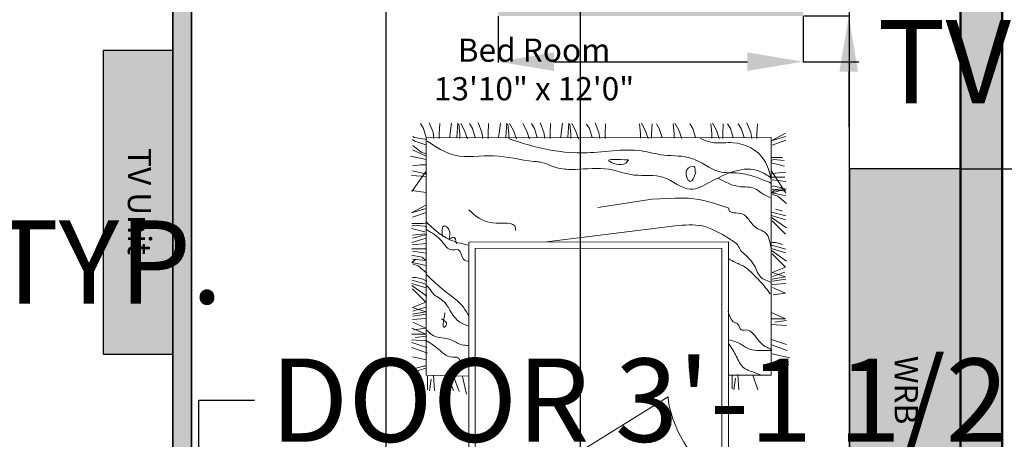
# Model space of a CAD drawing. Units: inches. Extents: x 2796 to 3603, y 978 to 1787.
# Tile 13 of 15: x 3212 to 3425, y 1545 to 1636. Entities that reach past the tile are written whole.
import ezdxf

# ---------------------------------------------------------------- set-up
doc = ezdxf.new("R2010")
doc.units = ezdxf.units.IN
for name, color, linetype, lineweight in [('A-ANNO-DIMS', 7, 'Continuous', 18), ('A-ANNO-TEXT', 7, 'Continuous', 18), ('A-AREA-IDEN', 7, 'Continuous', 18), ('A-FLOR-CASE', 2, 'Continuous', 25), ('A-FLOR-CASE-PATT', 2, 'Continuous', 13), ('A-WALL-EXTR-PATT', 1, 'Continuous', 13), ('A-WALL-INTR-PATT', 5, 'Continuous', 13), ('Furniture', 2, 'Continuous', 18), ('Inner Wall', 5, 'Continuous', 35), ('Outer Wall', 1, 'Continuous', 50)]:
    doc.layers.add(name, color=color, linetype=linetype, lineweight=lineweight)
doc.styles.get("Standard").update_dxf_attribs({"font": 'arial.ttf'})
doc.dimstyles.get("Standard").update_dxf_attribs({"dimtxt": 18, "dimasz": 12, "dimexe": 0.18, "dimexo": 0.0625, "dimgap": 0.09, "dimtad": 0, "dimtih": 1, "dimtoh": 1, "dimdec": 0, "dimzin": 0, "dimdsep": 46, "dimlunit": 3, "dimtxsty": 'Standard', "dimcen": 0.09, "dimadec": 0, "dimazin": 0, "dimtfac": 1, "dimtdec": 0, "dimtofl": 0, "dimtmove": 0, "dimatfit": 3, "dimfxl": 1, "dimtolj": 1, "dimtzin": 0, "dimarcsym": 0})

# ---------------------------------------------------------------- blocks, each defined once
blk = doc.blocks.new('A$C2B723114')
for p, q in [((0, 2.9047), (2.8274, 2.9047)), ((0, 2.8487), (0, 2.9047)), ((0.4243, 2.8697), (0.4243, 2.4855)), ((2.4742, 2.8697), (2.4742, 2.4855)), ((2.8274, 2.9047), (2.8274, 2.8487)), ((2.8274, 2.8487), (0, 2.8487)), ((0.1012, 2.4649), (0.1012, 2.849)), ((0.1396, 2.5033), (0.1396, 2.849)), ((0.6794, 0.7051), (0.6794, 2.8509)), ((0.7187, 0.7435), (0.7187, 2.8509)), ((2.1776, 2.8509), (2.1776, 0.7454)), ((2.216, 2.8509), (2.216, 0.707)), ((2.6798, 2.5052), (2.6798, 2.8509)), ((2.7182, 2.4668), (2.7182, 2.8509)), ((0.6087, 2.6776), (0.295, 2.6776)), ((2.6586, 2.6776), (2.2821, 2.6776)), ((1.3789, 2.4999), (1.3598, 2.5761)), ((2.0593, 2.4999), (2.0402, 2.5761)), ((2.2188, 2.5052), (2.6798, 2.5052)), ((0.6794, 2.4649), (0.1012, 2.4649)), ((0.6766, 2.5033), (0.1396, 2.5033)), ((0.7191, 2.47), (2.1778, 2.4719)), ((1.3858, 2.4723), (1.3789, 2.4999)), ((2.0662, 2.4723), (2.0593, 2.4999)), ((2.2188, 2.4668), (2.7182, 2.4668)), ((2.1771, 2.3036), (0.718, 2.1685)), ((1.0365, 1.6233), (2.1246, 2.2989)), ((0.5047, 1.5819), (0.5353, 1.4945)), ((0.6174, 1.5819), (0.6232, 1.4916)), ((0.6467, 1.5819), (0.6369, 1.5137)), ((0.6571, 1.4945), (0.6571, 1.5765)), ((2.2287, 1.6076), (2.2523, 1.5035)), ((2.2726, 1.593), (2.3061, 1.5007)), ((2.3067, 1.5881), (2.3373, 1.5007)), ((2.4194, 1.5881), (2.4251, 1.4979)), ((2.4487, 1.5881), (2.4389, 1.5199)), ((2.4591, 1.5007), (2.4591, 1.5828)), ((0.4269, 0.0884), (0.4269, 1.4945)), ((0.4269, 1.4945), (0.6794, 1.4945)), ((2.4685, 1.4964), (2.216, 1.5022)), ((2.4685, 1.4964), (2.4685, 0.0903)), ((2.4685, 1.4044), (2.5491, 1.3861)), ((0.3172, 1.3923), (0.4213, 1.3687)), ((0.3318, 1.3485), (0.4241, 1.3149)), ((2.4596, 1.3659), (2.552, 1.3324)), ((0.3367, 1.3143), (0.4241, 1.2838)), ((2.4645, 1.3318), (2.552, 1.3012)), ((2.4645, 1.2928), (2.5548, 1.2871)), ((2.4645, 1.2635), (2.5328, 1.2733)), ((2.4699, 1.2531), (2.552, 1.2163)), ((2.552, 1.2531), (2.4699, 1.2531)), ((2.5435, 1.2276), (2.4699, 1.2163)), ((0.3367, 1.2016), (0.427, 1.1959)), ((0.3367, 1.1724), (0.405, 1.1821)), ((2.5491, 1.1654), (2.467, 1.1597)), ((2.4699, 1.2163), (2.5463, 1.1823)), ((0.4241, 1.162), (0.3421, 1.162)), ((0.3421, 1.162), (0.4241, 1.1252)), ((2.5463, 1.1455), (2.467, 1.1342)), ((2.5491, 1.1342), (2.4699, 1.1201)), ((2.4699, 1.1201), (2.5491, 1.0946)), ((2.5463, 1.1172), (2.4727, 1.0918)), ((2.5491, 1.0946), (2.4699, 1.0635)), ((2.4699, 1.0635), (2.5491, 0.9842)), ((0.4157, 1.0206), (0.3421, 1.0093)), ((0.3421, 1.0093), (0.4185, 0.9754)), ((2.4642, 1.0267), (2.552, 0.9644)), ((0.4213, 0.9584), (0.3392, 0.9527)), ((0.4185, 0.9386), (0.3392, 0.9272)), ((2.4642, 0.9389), (2.4869, 0.9276)), ((2.467, 0.9559), (2.552, 0.9333)), ((2.4699, 0.9785), (2.552, 0.9531)), ((0.4213, 0.9272), (0.3421, 0.9131)), ((0.3421, 0.9131), (0.4213, 0.8876)), ((0.4213, 0.8876), (0.3421, 0.8565)), ((0.4185, 0.9103), (0.3449, 0.8848)), ((2.4642, 0.8908), (2.5152, 0.8483)), ((2.4869, 0.9276), (2.5265, 0.9163)), ((2.5265, 0.9163), (2.5491, 0.9163)), ((0.3364, 0.8197), (0.4241, 0.7574)), ((0.3421, 0.8565), (0.4213, 0.7772)), ((2.467, 0.8455), (2.5208, 0.8342)), ((2.4699, 0.8172), (2.4925, 0.7974)), ((2.5491, 0.8087), (2.4699, 0.8172)), ((2.5152, 0.8483), (2.5491, 0.837)), ((2.5208, 0.8342), (2.552, 0.8285)), ((2.552, 0.8285), (2.5293, 0.8087)), ((0.3421, 0.7716), (0.4241, 0.7461)), ((2.5491, 0.7606), (2.467, 0.7719)), ((2.4925, 0.7974), (2.535, 0.7889)), ((2.535, 0.7889), (2.552, 0.7861)), ((0.3392, 0.7489), (0.4241, 0.7263)), ((0.359, 0.7206), (0.3987, 0.7093)), ((0.3987, 0.7093), (0.4213, 0.7093)), ((2.216, 0.707), (0.6794, 0.7051)), ((2.1776, 0.7454), (0.7187, 0.7435)), ((0.9938, 0.6115), (1.7555, 0.7064)), ((2.4727, 0.7464), (2.467, 0.7408)), ((2.467, 0.7153), (2.5491, 0.7238)), ((2.552, 0.7096), (2.467, 0.6842)), ((2.552, 0.7464), (2.4727, 0.7464)), ((0.3421, 0.6601), (0.4213, 0.5808)), ((2.5491, 0.6842), (2.4642, 0.6615)), ((2.5491, 0.6672), (2.4755, 0.6587)), ((2.4755, 0.6474), (2.5548, 0.6276)), ((0.3364, 0.6233), (0.4241, 0.561)), ((2.4642, 0.6191), (2.4784, 0.6134)), ((2.467, 0.5993), (2.4869, 0.5964)), ((2.4784, 0.6134), (2.5406, 0.6077)), ((2.4869, 0.5964), (2.552, 0.5964)), ((2.5406, 0.6077), (2.552, 0.6134)), ((0.3392, 0.5525), (0.4241, 0.5299)), ((0.3421, 0.5752), (0.4241, 0.5497)), ((2.467, 0.5313), (2.5491, 0.5596)), ((2.467, 0.5087), (2.5548, 0.5342)), ((2.5548, 0.5342), (2.4699, 0.4889)), ((0.3364, 0.4785), (0.3874, 0.436)), ((0.359, 0.5242), (0.3987, 0.5129)), ((1.4523, 0.5021), (1.1305, 0.4537)), ((0.4213, 0.415), (0.3364, 0.3923)), ((0.3392, 0.4332), (0.393, 0.4219)), ((0.4241, 0.2868), (0.3392, 0.415)), ((0.3874, 0.436), (0.4213, 0.4247)), ((0.393, 0.4219), (0.4241, 0.4162)), ((0.4241, 0.4162), (0.4015, 0.3964)), ((1.1305, 0.4537), (0.9938, 0.448)), ((2.467, 0.4133), (2.552, 0.4019)), ((0.3421, 0.4049), (0.3647, 0.3851)), ((0.4213, 0.3964), (0.3421, 0.4049)), ((0.4213, 0.398), (0.3477, 0.3895)), ((0.3647, 0.3851), (0.4072, 0.3766)), ((0.4072, 0.3766), (0.4241, 0.3738)), ((2.467, 0.2879), (2.552, 0.4076)), ((0.4213, 0.3377), (0.3392, 0.3491)), ((0.3392, 0.2925), (0.4213, 0.3009)), ((0.4241, 0.3236), (0.3449, 0.3236)), ((2.4642, 0.3049), (2.5491, 0.2851)), ((2.467, 0.319), (2.5548, 0.3134)), ((0.3477, 0.2571), (0.427, 0.2373)), ((2.4699, 0.2491), (2.501, 0.2491)), ((2.501, 0.2491), (2.5491, 0.2547)), ((0.3506, 0.2231), (0.4128, 0.2175)), ((0.359, 0.2061), (0.4241, 0.2061)), ((0.4128, 0.2175), (0.4241, 0.2231)), ((2.467, 0.2179), (2.5605, 0.1981)), ((2.467, 0.1981), (2.5491, 0.1613)), ((2.467, 0.184), (2.4982, 0.1755)), ((2.4982, 0.1755), (2.5463, 0.1359)), ((0.3392, 0.1042), (0.4213, 0.1325)), ((2.4699, 0.1302), (2.535, 0.1104)), ((0.3392, 0.0815), (0.427, 0.107)), ((0.427, 0.107), (0.3421, 0.0617)), ((2.4685, 0.0903), (0.4269, 0.0884)), ((0.5106, 0.0657), (0.5077, 0.0063)), ((0.5106, 0.094), (0.5106, 0.0657)), ((0.5417, 0.094), (0.5474, 0.0572)), ((0.587, 0.0884), (0.604, 0.0346)), ((0.6512, 0.0884), (0.6682, 0.0346)), ((0.713, 0.0657), (0.7101, 0.0063)), ((0.713, 0.094), (0.713, 0.0657)), ((0.7334, 0.0943), (0.7503, 0.0434)), ((0.7786, 0.0915), (0.7786, 0.0632)), ((0.7786, 0.0632), (0.7843, 0.0066)), ((0.8739, 0.0884), (0.8908, 0.0346)), ((0.956, 0.0943), (0.973, 0.0434)), ((1.0013, 0.0915), (1.0013, 0.0632)), ((1.0013, 0.0632), (1.007, 0.0066)), ((1.072, 0.0884), (1.089, 0.0346)), ((1.1338, 0.0657), (1.131, 0.0063)), ((1.1338, 0.094), (1.1338, 0.0657)), ((1.1542, 0.0943), (1.1712, 0.0434)), ((1.1995, 0.0915), (1.1995, 0.0632)), ((1.1995, 0.0632), (1.2052, 0.0066)), ((1.4088, 0.0657), (1.406, 0.0063)), ((1.4088, 0.094), (1.4088, 0.0657)), ((1.44, 0.094), (1.4456, 0.0572)), ((1.4853, 0.0884), (1.5023, 0.0346)), ((1.5674, 0.0962), (1.5844, 0.0453)), ((1.6127, 0.0934), (1.6127, 0.0651)), ((1.6127, 0.0651), (1.6184, 0.0085)), ((1.6297, 0.0849), (1.624, 0.0028)), ((1.6693, 0.0623), (1.6608, 0.0028)), ((1.6721, 0.0877), (1.6693, 0.0623)), ((1.7344, 0.0651), (1.7316, 0.0057)), ((1.7344, 0.0934), (1.7344, 0.0651)), ((1.7655, 0.0934), (1.7712, 0.0566)), ((1.8108, 0.0877), (1.8278, 0.034)), ((1.8568, 0.0962), (1.8738, 0.0453)), ((1.9342, 0.0962), (1.9512, 0.0453)), ((1.9795, 0.0934), (1.9795, 0.0651)), ((1.9795, 0.0651), (1.9852, 0.0085)), ((1.9965, 0.0849), (1.9908, 0.0028)), ((2.0361, 0.0623), (2.0276, 0.0028)), ((2.039, 0.0877), (2.0361, 0.0623)), ((2.1012, 0.0651), (2.0984, 0.0057)), ((2.1012, 0.0934), (2.1012, 0.0651)), ((2.1324, 0.0934), (2.138, 0.0566)), ((2.1777, 0.0877), (2.1946, 0.034)), ((2.2236, 0.0962), (2.2406, 0.0453)), ((2.2689, 0.0934), (2.2689, 0.0651)), ((2.2689, 0.0651), (2.2746, 0.0085)), ((2.2859, 0.0849), (2.2802, 0.0028)), ((2.3255, 0.0623), (2.317, 0.0028)), ((2.3284, 0.0877), (2.3255, 0.0623)), ((2.3906, 0.0651), (2.3878, 0.0057)), ((2.3906, 0.0934), (2.3906, 0.0651)), ((2.4218, 0.0934), (2.4274, 0.0566)), ((2.4642, 0.0991), (2.5378, 0.0877)), ((2.467, 0.0877), (2.484, 0.034)), ((2.535, 0.1104), (2.5491, 0.0991)), ((2.5378, 0.0877), (2.5463, 0.0821)), ((0.5474, 0.0572), (0.57, 0.0006)), ((0.604, 0.0346), (0.621, 0.0063)), ((0.6682, 0.0346), (0.6851, 0.0063)), ((0.7503, 0.0434), (0.773, 0.0037)), ((0.8908, 0.0346), (0.9078, 0.0063)), ((0.973, 0.0434), (0.9957, 0.0037)), ((1.089, 0.0346), (1.106, 0.0063)), ((1.1712, 0.0434), (1.1939, 0.0037)), ((1.4456, 0.0572), (1.4683, 0.0006)), ((1.5023, 0.0346), (1.5192, 0.0082)), ((1.5844, 0.0453), (1.607, 0.0057)), ((1.7712, 0.0566), (1.7938, 0)), ((1.8278, 0.034), (1.8448, 0.0057)), ((1.8738, 0.0453), (1.8964, 0.0057)), ((1.9512, 0.0453), (1.9739, 0.0057)), ((2.138, 0.0566), (2.1607, 0)), ((2.1946, 0.034), (2.2116, 0.0057)), ((2.2406, 0.0453), (2.2632, 0.0057)), ((2.4274, 0.0566), (2.4501, 0)), ((2.484, 0.034), (2.501, 0.0057))]:
    blk.add_line(p, q)
for centre, radius in [((0.4243, 2.6776), 0.0821), ((2.4742, 2.6776), 0.0821), ((0.4243, 2.6776), 0.0493), ((2.4742, 2.6776), 0.0493)]:
    blk.add_circle(centre, radius)
for centre, radius, start, end in [((0.8078, 2.821), 0.00214, 160.43603, 281.89306), ((0.8088, 2.8207), 0.00315, 111.7883, 160.43603), ((0.8162, 2.8021), 0.0232, 94.30254, 111.7883), ((0.8091, 2.8151), 0.00394, 21.9904, 101.89306), ((0.8409, 2.7949), 0.0302, 158.57902, 188.13348), ((0.7994, 2.8112), 0.0144, 338.57902, 21.9904), ((0.8165, 2.7987), 0.0266, 59.34875, 94.30254), ((0.8554, 2.8643), 0.0497, 239.34875, 264.74081), ((0.9202, 3.5684), 0.7568, 264.74081, 268.09211), ((0.8679, 2.7254), 0.0915, 74.06476, 94.21588), ((0.8679, 2.7254), 0.0915, 53.91364, 74.06476), ((0.9409, 4.189), 1.3777, 268.09211, 270.57574), ((0.8679, 2.7254), 0.0915, 36.17665, 53.91364), ((0.86, 2.6097), 0.2158, 62.76041, 69.13972), ((0.9466, 3.6164), 0.8051, 270.57574, 274.80185), ((0.9263, 2.7386), 0.0708, 51.61143, 62.76041), ((1.0364, 2.548), 0.2671, 87.46141, 94.80185), ((1.042, 2.6745), 0.1405, 79.81012, 87.46141), ((1.1532, 3.2931), 0.488, 259.81012, 263.9133), ((1.204, 3.7695), 0.9671, 263.9133, 270), ((1.204, 3.4318), 0.6294, 270, 277.54685), ((1.2573, 3.0292), 0.2233, 277.54685, 285.74398), ((1.3941, 2.5438), 0.281, 98.43719, 105.74398), ((1.3747, 2.6748), 0.1486, 90, 98.43719), ((1.3713, 2.8186), 0.0315, 274.40021, 333.41948), ((1.3747, 2.74), 0.0833, 78.72762, 90), ((1.3886, 2.8099), 0.0121, 333.41948, 78.72762), ((1.4882, 2.821), 0.00214, 160.43603, 281.89306), ((1.4892, 2.8207), 0.00315, 111.7883, 160.43603), ((1.4966, 2.8021), 0.0232, 94.30254, 111.7883), ((1.4895, 2.8151), 0.00394, 21.9904, 101.89306), ((1.5213, 2.7949), 0.0302, 158.57902, 188.13348), ((1.4798, 2.8112), 0.0144, 338.57902, 21.9904), ((1.4969, 2.7987), 0.0266, 59.34875, 94.30254), ((1.5358, 2.8643), 0.0497, 239.34875, 264.74081), ((1.6006, 3.5684), 0.7568, 264.74081, 268.09211), ((1.5483, 2.7254), 0.0915, 74.06476, 94.21588), ((1.5483, 2.7254), 0.0915, 53.91364, 74.06476), ((1.6213, 4.189), 1.3777, 268.09211, 270.57574), ((1.5483, 2.7254), 0.0915, 36.17665, 53.91364), ((1.5404, 2.6097), 0.2158, 62.76041, 69.13972), ((1.627, 3.6164), 0.8051, 270.57574, 274.80185), ((1.6067, 2.7386), 0.0708, 51.61143, 62.76041), ((1.7168, 2.548), 0.2671, 87.46141, 94.80185), ((1.7224, 2.6745), 0.1405, 79.81012, 87.46141), ((1.8336, 3.2931), 0.488, 259.81012, 263.9133), ((1.8844, 3.7695), 0.9671, 263.9133, 270), ((1.8844, 3.4318), 0.6294, 270, 277.54685), ((1.9377, 3.0292), 0.2233, 277.54685, 285.74398), ((2.0745, 2.5438), 0.281, 98.43719, 105.74398), ((2.0551, 2.6748), 0.1486, 90, 98.43719), ((2.0517, 2.8186), 0.0315, 274.40021, 333.41948), ((2.0551, 2.74), 0.0833, 78.72762, 90), ((2.069, 2.8099), 0.0121, 333.41948, 78.72762), ((1.0356, 2.8227), 0.2268, 188.13348, 192.10946), ((0.635, 2.7368), 0.1829, 7.6809, 12.10946), ((-0.0181, 2.6487), 0.8418, 3.36875, 7.6809), ((0.8679, 2.7254), 0.0915, 18.43965, 36.17665), ((0.7461, 2.511), 0.3611, 46.18849, 51.61143), ((0.8523, 2.6218), 0.2076, 39.03494, 46.18849), ((0.9783, 2.7239), 0.0455, 28.31676, 39.03494), ((0.8558, 2.6579), 0.1846, 23.00277, 28.31676), ((0.923, 2.7382), 0.4535, 0, 6.23236), ((1.1884, 2.7382), 0.1881, 350.31563, 0), ((1.716, 2.8227), 0.2268, 188.13348, 192.10946), ((1.3154, 2.7368), 0.1829, 7.6809, 12.10946), ((0.6623, 2.6487), 0.8418, 3.36875, 7.6809), ((1.5483, 2.7254), 0.0915, 18.43965, 36.17665), ((1.4265, 2.511), 0.3611, 46.18849, 51.61143), ((1.5327, 2.6218), 0.2076, 39.03494, 46.18849), ((1.6587, 2.7239), 0.0455, 28.31676, 39.03494), ((1.5362, 2.6579), 0.1846, 23.00277, 28.31676), ((1.6034, 2.7382), 0.4535, 0, 6.23236), ((1.8688, 2.7382), 0.1881, 350.31563, 0), ((0.1976, 2.6614), 0.6258, 358.36691, 3.36875), ((0.5722, 2.8434), 0.8132, 347.80162, 350.31563), ((0.878, 2.6614), 0.6258, 358.36691, 3.36875), ((1.2526, 2.8434), 0.8132, 347.80162, 350.31563), ((-0.4351, 2.6794), 1.2587, 356.94504, 358.36691), ((1.9648, 2.5659), 0.6074, 171.99495, 177.33512), ((1.6528, 2.6098), 0.2924, 167.80162, 171.99495), ((0.2453, 2.6794), 1.2587, 356.94504, 358.36691), ((2.6452, 2.5659), 0.6074, 171.99495, 177.33512), ((2.3332, 2.6098), 0.2924, 167.80162, 171.99495), ((-11.7321, 3.2823), 12.5718, 356.49514, 356.94504), ((1.4204, 2.5912), 0.0624, 177.33512, 194.04519), ((-11.0517, 3.2823), 12.5718, 356.49514, 356.94504), ((2.1008, 2.5912), 0.0624, 177.33512, 194.04519), ((0.5206, 2.5319), 0.2961, 350.00164, 356.49514), ((1.4917, 3.1364), 0.681, 244.68893, 246.51559), ((1.4917, 3.1364), 0.681, 246.51559, 248.34226), ((1.201, 2.5319), 0.2961, 350.00164, 356.49514), ((2.1721, 3.1364), 0.681, 244.68893, 246.51559), ((2.1721, 3.1364), 0.681, 246.51559, 248.34226), ((0.8298, 2.4774), 0.0178, 170.00164, 196.69777), ((0.8139, 2.4726), 0.00122, 196.69777, 277.12039), ((0.8041, 2.5514), 0.0807, 277.12039, 286.22115), ((0.8068, 2.5419), 0.0707, 286.22115, 297.28412), ((0.8584, 2.4419), 0.0418, 102.86904, 117.28412), ((0.879, 2.3515), 0.1345, 93.57397, 102.86904), ((0.9376, 1.4146), 1.0732, 90.28654, 93.57397), ((0.9586, -2.7845), 5.2724, 89.02962, 90.28654), ((0.9954, -0.6123), 3.0999, 87.39037, 89.02962), ((1.0854, 1.364), 1.1216, 85.38242, 87.39037), ((1.28, 3.7729), 1.2952, 265.38242, 267.25094), ((1.228, 2.691), 0.2121, 267.25094, 281.55856), ((1.4917, 3.1364), 0.681, 248.34226, 250.57202), ((1.4917, 3.1364), 0.681, 250.57202, 252.80178), ((1.2975, 2.3514), 0.1345, 83.56595, 101.55856), ((1.3002, 2.3754), 0.1104, 72.61359, 83.56595), ((1.3965, 2.6828), 0.2118, 252.61359, 260.5159), ((1.4027, 2.7202), 0.2496, 260.5159, 265.91706), ((1.385, 2.4721), 0.000845, 265.91706, 14.04494), ((1.5102, 2.4774), 0.0178, 170.00164, 196.69777), ((1.4943, 2.4726), 0.00122, 196.69777, 277.12039), ((1.4845, 2.5514), 0.0807, 277.12039, 286.22115), ((1.4872, 2.5419), 0.0707, 286.22115, 297.28412), ((1.5388, 2.4419), 0.0418, 102.86904, 117.28412), ((1.5594, 2.3515), 0.1345, 93.57397, 102.86904), ((1.618, 1.4146), 1.0732, 90.28654, 93.57397), ((1.639, -2.7845), 5.2724, 89.02962, 90.28654), ((1.6758, -0.6123), 3.0999, 87.39037, 89.02962), ((1.7658, 1.364), 1.1216, 85.38242, 87.39037), ((1.9604, 3.7729), 1.2952, 265.38242, 267.25094), ((1.9084, 2.691), 0.2121, 267.25094, 281.55856), ((2.1721, 3.1364), 0.681, 248.34226, 250.57202), ((2.1721, 3.1364), 0.681, 250.57202, 252.80178), ((1.9779, 2.3514), 0.1345, 83.56595, 101.55856), ((1.9806, 2.3754), 0.1104, 72.61359, 83.56595), ((2.0769, 2.6828), 0.2118, 252.61359, 260.5159), ((2.0831, 2.7202), 0.2496, 260.5159, 265.91706), ((2.0654, 2.4721), 0.000845, 265.91706, 14.04494)]:
    blk.add_arc(centre, radius, start, end)
blk.add_ellipse((0.4962, 1.9132), major_axis=(0.4887, -0.4605), ratio=0.503305, start_param=0.491272, end_param=1.591113)
for points, knots in [([(0.427, 1.4678), (0.4036, 1.4582), (0.3693, 1.4441), (0.3335, 1.4344), (0.3221, 1.4313)], [0, 0, 0, 0, 98.452083, 144.639601, 144.639601, 144.639601, 144.639601]), ([(0.6768, 1.3104), (0.6615, 1.3339), (0.6315, 1.3797), (0.604, 1.4501), (0.5417, 1.4748), (0.5064, 1.4871), (0.4848, 1.4945)], [0, 0, 0, 0, 110.980521, 216.571322, 273.316778, 363.252298, 363.252298, 363.252298, 363.252298]), ([(2.5548, 1.4853), (2.5314, 1.4757), (2.5031, 1.4641), (2.4737, 1.4555), (2.4685, 1.454)], [0, 0, 0, 0, 98.452083, 119.481049, 119.481049, 119.481049, 119.481049]), ([(2.552, 1.4598), (2.5309, 1.4545), (2.5031, 1.4475), (2.4753, 1.4406), (2.4685, 1.4389)], [0, 0, 0, 0, 84.638756, 111.94623, 111.94623, 111.94623, 111.94623]), ([(0.4241, 1.4423), (0.4031, 1.437), (0.3691, 1.4284), (0.3351, 1.4199), (0.3221, 1.4167)], [0, 0, 0, 0, 84.638756, 136.955563, 136.955563, 136.955563, 136.955563]), ([(2.2145, 1.4211), (2.233, 1.4246), (2.2636, 1.4303), (2.2761, 1.3837), (2.3429, 1.3967), (2.3949, 1.3342), (2.4474, 1.3031), (2.4698, 1.2898)], [0, 0, 0, 0, 61.886907, 102.717887, 145.699352, 284.082577, 386.765171, 386.765171, 386.765171, 386.765171]), ([(0.6768, 1.286), (0.6567, 1.2911), (0.6145, 1.3017), (0.5543, 1.3533), (0.4816, 1.349), (0.4362, 1.3493), (0.4233, 1.3493)], [0, 0, 0, 0, 80.250278, 168.388677, 295.908361, 346.663112, 346.663112, 346.663112, 346.663112]), ([(0.4233, 1.3445), (0.4367, 1.3385), (0.464, 1.3264), (0.5129, 1.2848), (0.5456, 1.2161), (0.6131, 1.2349), (0.6142, 1.1913), (0.6642, 1.1806), (0.674, 1.144), (0.6817, 1.1154)], [0, 0, 0, 0, 56.745495, 115.23739, 254.956954, 286.678662, 337.828324, 366.201072, 468.500395, 468.500395, 468.500395, 468.500395]), ([(2.2145, 1.319), (2.2295, 1.319), (2.2678, 1.3192), (2.3288, 1.2705), (2.4143, 1.279), (2.4535, 1.2403), (2.4662, 1.2278)], [0, 0, 0, 0, 57.155505, 146.33427, 287.936209, 355.396728, 355.396728, 355.396728, 355.396728]), ([(2.3573, 1.127), (2.3656, 1.1759), (2.3758, 1.2352), (2.3371, 1.1853), (2.3602, 1.1713), (2.3768, 1.1612)], [0, 0, 0, 0, 107.853607, 130.728419, 189.220329, 189.220329, 189.220329, 189.220329]), ([(2.2182, 1.2059), (2.2419, 1.1958), (2.3116, 1.1659), (2.342, 1.0552), (2.4266, 1.0223), (2.4474, 0.9811), (2.462, 0.9684), (2.4698, 0.9616)], [0, 0, 0, 0, 97.73655, 287.59661, 389.176293, 423.403759, 463.679181, 463.679181, 463.679181, 463.679181]), ([(2.2145, 1.1476), (2.2246, 1.1286), (2.2575, 1.0666), (2.3612, 1.0009), (2.431, 0.9336), (2.4662, 0.8996)], [0, 0, 0, 0, 83.02987, 271.460712, 463.033803, 463.033803, 463.033803, 463.033803]), ([(0.6817, 0.8034), (0.6673, 0.8119), (0.6341, 0.8315), (0.5785, 0.8518), (0.5349, 0.8973), (0.4828, 0.9461), (0.4518, 0.9879), (0.4331, 1.013)], [0, 0, 0, 0, 65.318952, 150.437229, 226.833166, 307.58338, 429.454095, 429.454095, 429.454095, 429.454095]), ([(0.4282, 0.9448), (0.4547, 0.9353), (0.496, 0.9206), (0.5223, 0.8436), (0.5628, 0.7946), (0.6113, 0.7575), (0.6214, 0.7173), (0.6539, 0.7022), (0.672, 0.6897), (0.6768, 0.6864)], [0, 0, 0, 0, 102.299436, 159.044876, 303.717955, 348.579152, 391.138254, 454.581655, 477.456496, 477.456496, 477.456496, 477.456496]), ([(2.2145, 0.823), (2.227, 0.8201), (2.261, 0.8121), (2.261, 0.7401), (2.3352, 0.7659), (2.379, 0.6836), (2.4336, 0.6521), (2.4662, 0.6334)], [0, 0, 0, 0, 46.747668, 127.438174, 179.649794, 280.561838, 429.605131, 429.605131, 429.605131, 429.605131]), ([(0.4282, 0.74), (0.4347, 0.7029), (0.444, 0.6496), (0.5194, 0.6274), (0.555, 0.5807), (0.5975, 0.5243), (0.6789, 0.5415), (0.677, 0.5095), (0.6768, 0.5061)], [0, 0, 0, 0, 130.791737, 187.537266, 286.231946, 353.673191, 460.023761, 472.712403, 472.712403, 472.712403, 472.712403]), ([(2.2218, 0.7246), (2.2595, 0.716), (2.3548, 0.6945), (2.4265, 0.6268), (2.4698, 0.586)], [0, 0, 0, 0, 148.665024, 375.555892, 375.555892, 375.555892, 375.555892]), ([(2.3719, 0.6737), (2.3738, 0.6431), (2.3772, 0.5878), (2.3146, 0.6382), (2.3401, 0.7015), (2.2971, 0.6649), (2.2923, 0.6965), (2.289, 0.7176)], [0, 0, 0, 0, 83.446591, 150.887818, 201.642461, 230.015204, 286.760644, 286.760644, 286.760644, 286.760644]), ([(0.6768, 0.6864), (0.7275, 0.655), (0.8251, 0.5944), (0.9391, 0.606), (0.9938, 0.6115)], [0, 0, 0, 0, 225.995823, 434.686543, 434.686543, 434.686543, 434.686543]), ([(2.2145, 0.5167), (2.1764, 0.5522), (2.1051, 0.6184), (1.9357, 0.5803), (1.9385, 0.6342), (1.9388, 0.6395)], [0, 0, 0, 0, 208.073343, 389.01094, 409.01094, 409.01094, 409.01094, 409.01094]), ([(0.6768, 0.5061), (0.7554, 0.4794), (0.8591, 0.4442), (0.9675, 0.4473), (0.9938, 0.448)], [0, 0, 0, 0, 319.374611, 421.61723, 421.61723, 421.61723, 421.61723]), ([(0.4331, 0.4427), (0.4498, 0.4356), (0.4827, 0.4216), (0.5314, 0.3759), (0.632, 0.3884), (0.6996, 0.3513), (0.7423, 0.3278)], [0, 0, 0, 0, 70.931849, 139.556414, 248.154027, 434.709995, 434.709995, 434.709995, 434.709995]), ([(2.4625, 0.1088), (2.4095, 0.1438), (2.2904, 0.2226), (2.0623, 0.1771), (1.9006, 0.2246), (1.7699, 0.2337), (1.6941, 0.2766), (1.5528, 0.2786), (1.4005, 0.2587), (1.2324, 0.3267), (1.059, 0.2939), (0.9218, 0.426), (0.7359, 0.3204), (0.5586, 0.2391), (0.4502, 0.3116), (0.427, 0.3272)], [0, 0, 0, 0, 239.874704, 538.942419, 850.40885, 893.390315, 1047.998294, 1176.505142, 1437.500972, 1637.333004, 1864.324391, 2089.058767, 2248.736533, 2637.953392, 2744.252142, 2744.252142, 2744.252142, 2744.252142]), ([(1.9771, 0.0962), (1.9286, 0.1117), (1.7864, 0.157), (1.5223, 0.1992), (1.2611, 0.141), (1.0527, 0.2023), (0.8859, 0.1885), (0.76, 0.3042), (0.6211, 0.292), (0.5187, 0.3203), (0.4572, 0.3456), (0.4282, 0.3575)], [0, 0, 0, 0, 198.710624, 582.73994, 1031.873213, 1206.082894, 1423.278209, 1655.952104, 1808.744089, 1945.69963, 2068.229211, 2068.229211, 2068.229211, 2068.229211]), ([(0.8718, 0.2941), (0.8821, 0.3221), (0.9041, 0.3814), (0.9523, 0.2773), (0.8733, 0.2454), (0.8757, 0.2798), (0.8766, 0.2941)], [0, 0, 0, 0, 82.720021, 175.094899, 237.579423, 282.440623, 282.440623, 282.440623, 282.440623]), ([(0.8474, 0.0943), (0.82, 0.1047), (0.757, 0.1287), (0.6201, 0.1029), (0.4623, 0.1837), (0.4372, 0.2936), (0.4282, 0.3331)], [0, 0, 0, 0, 112.422038, 258.341957, 533.791494, 688.286079, 688.286079, 688.286079, 688.286079]), ([(1.2715, 0.221), (1.3344, 0.2172), (1.4529, 0.21), (1.2971, 0.2665), (1.2756, 0.2284), (1.2715, 0.221)], [0, 0, 0, 0, 150.888188, 283.977876, 315.699589, 315.699589, 315.699589, 315.699589])]:
    blk.add_open_spline(points, degree=3, knots=knots)
blk = doc.blocks.new('TV-UNIT-66IN-NOM')
blk.add_lwpolyline([(0, 0), (65.77, 0), (65.77, -15), (0, -15)], close=True)
blk = doc.blocks.new('*D18')
at = {"layer": 'A-ANNO-DIMS', "color": 0, "lineweight": -2, "transparency": 16777216}
for p, q in [((3250.87, 1541.68), (3250.87, 1553.68)), ((3250.87, 1553.68), (3262.87, 1553.68)), ((3245.31, 1541.68), (3251.05, 1541.68)), ((3250.87, 1516.18), (3250.87, 1529.68)), ((3245.31, 1504.18), (3251.05, 1504.18))]:
    blk.add_line(p, q, dxfattribs=at)
at = {"layer": 'A-ANNO-DIMS', "color": 0, "transparency": 16777216}
for points in [[(3248.87, 1529.68), (3252.87, 1529.68), (3250.87, 1541.68)], [(3248.87, 1516.18), (3252.87, 1516.18), (3250.87, 1504.18)]]:
    blk.add_solid(points, dxfattribs=at)
at = {"layer": 'Defpoints', "color": 0, "transparency": 16777216}
for p in [(3245.25, 1541.68), (3250.87, 1541.68), (3245.25, 1504.18)]:
    blk.add_point(p, dxfattribs=at)
at = {"layer": 'A-ANNO-DIMS', "color": 0, "transparency": 16777216, "insert": (3379.56, 1553.68), "char_height": 18, "attachment_point": 5}
blk.add_mtext('\\A1;DOOR 3\'-1 1/2" TYP.', dxfattribs=at)
blk = doc.blocks.new('*D20')
at = {"layer": 'A-ANNO-DIMS', "color": 0, "lineweight": -2, "transparency": 16777216}
for p, q in [((3277.07, 1677.68), (3277.07, 1689.68)), ((3277.07, 1689.68), (3289.07, 1689.68)), ((3273.31, 1677.68), (3277.25, 1677.68)), ((3277.07, 1664.18), (3277.07, 1665.68)), ((3273.31, 1652.18), (3277.25, 1652.18))]:
    blk.add_line(p, q, dxfattribs=at)
at = {"layer": 'A-ANNO-DIMS', "color": 0, "transparency": 16777216}
for points in [[(3275.07, 1665.68), (3279.07, 1665.68), (3277.07, 1677.68)], [(3275.07, 1664.18), (3279.07, 1664.18), (3277.07, 1652.18)]]:
    blk.add_solid(points, dxfattribs=at)
at = {"layer": 'Defpoints', "color": 0, "transparency": 16777216}
for p in [(3273.25, 1677.68), (3277.07, 1677.68), (3273.25, 1652.18)]:
    blk.add_point(p, dxfattribs=at)
at = {"layer": 'A-ANNO-DIMS', "color": 0, "transparency": 16777216, "insert": (3405.76, 1689.68), "char_height": 18, "attachment_point": 5}
blk.add_mtext('\\A1;DOOR 2\'-1 1/2" TYP.', dxfattribs=at)
blk = doc.blocks.new('*D21')
at = {"layer": 'A-ANNO-DIMS', "color": 0, "lineweight": -2, "transparency": 16777216}
for p, q in [((3249.25, 1652.11), (3249.25, 1648.17)), ((3273.25, 1652.11), (3273.25, 1648.17)), ((3237.25, 1648.35), (3225.25, 1648.35)), ((3285.25, 1648.35), (3297.25, 1648.35))]:
    blk.add_line(p, q, dxfattribs=at)
at = {"layer": 'A-ANNO-DIMS', "color": 0, "transparency": 16777216}
for points in [[(3237.25, 1650.35), (3237.25, 1646.35), (3249.25, 1648.35)], [(3285.25, 1650.35), (3285.25, 1646.35), (3273.25, 1648.35)]]:
    blk.add_solid(points, dxfattribs=at)
at = {"layer": 'Defpoints', "color": 0, "transparency": 16777216}
for p in [(3249.25, 1652.18), (3273.25, 1652.18), (3273.25, 1648.35)]:
    blk.add_point(p, dxfattribs=at)
at = {"layer": 'A-ANNO-DIMS', "color": 0, "transparency": 16777216, "insert": (3352.35, 1648.35), "char_height": 18, "attachment_point": 5}
blk.add_mtext('\\A1;2\'-0" TYP.', dxfattribs=at)
blk = doc.blocks.new('*D27')
at = {"layer": 'A-ANNO-DIMS', "color": 0, "lineweight": -2, "transparency": 16777216}
for p, q in [((3185.26, 1635.1), (3201.27, 1635.1)), ((3201.09, 1623.1), (3201.09, 1592.81)), ((3201.09, 1543.97), (3201.09, 1574.25)), ((3185.26, 1531.97), (3201.27, 1531.97))]:
    blk.add_line(p, q, dxfattribs=at)
at = {"layer": 'A-ANNO-DIMS', "color": 0, "transparency": 16777216}
for points in [[(3199.09, 1623.1), (3203.09, 1623.1), (3201.09, 1635.1)], [(3199.09, 1543.97), (3203.09, 1543.97), (3201.09, 1531.97)]]:
    blk.add_solid(points, dxfattribs=at)
at = {"layer": 'Defpoints', "color": 0, "transparency": 16777216}
for p in [(3185.2, 1635.1), (3201.09, 1635.1), (3185.2, 1531.97)]:
    blk.add_point(p, dxfattribs=at)
at = {"layer": 'A-ANNO-DIMS', "color": 0, "transparency": 16777216, "insert": (3201.09, 1583.53), "char_height": 18, "attachment_point": 5}
blk.add_mtext('\\A1;8\'-7" TYP.', dxfattribs=at)
blk = doc.blocks.new('*D28')
at = {"layer": 'A-ANNO-DIMS', "color": 0, "lineweight": -2, "transparency": 16777216}
for p, q in [((3315.48, 1636.61), (3315.48, 1626.63)), ((3381.25, 1636.61), (3381.25, 1626.63)), ((3327.48, 1626.81), (3369.25, 1626.81)), ((3381.25, 1626.81), (3393.25, 1626.81))]:
    blk.add_line(p, q, dxfattribs=at)
at = {"layer": 'A-ANNO-DIMS', "color": 0, "transparency": 16777216}
for points in [[(3327.48, 1628.81), (3327.48, 1624.81), (3315.48, 1626.81)], [(3369.25, 1628.81), (3369.25, 1624.81), (3381.25, 1626.81)]]:
    blk.add_solid(points, dxfattribs=at)
at = {"layer": 'Defpoints', "color": 0, "transparency": 16777216}
for p in [(3315.48, 1636.68), (3381.25, 1636.68), (3381.25, 1626.81)]:
    blk.add_point(p, dxfattribs=at)
at = {"layer": 'A-ANNO-DIMS', "color": 0, "transparency": 16777216, "insert": (3500.81, 1626.81), "char_height": 18, "attachment_point": 5}
blk.add_mtext('\\A1;TV UNIT 5\'-6" TYP.', dxfattribs=at)
blk = doc.blocks.new('*D29')
at = {"layer": 'A-ANNO-DIMS', "color": 0, "lineweight": -2, "transparency": 16777216}
for p, q in [((3391.11, 1663.68), (3391.11, 1675.68)), ((3391.11, 1675.68), (3403.11, 1675.68)), ((3381.31, 1651.68), (3391.29, 1651.68)), ((3381.31, 1636.68), (3391.29, 1636.68)), ((3391.11, 1624.68), (3391.11, 1612.68))]:
    blk.add_line(p, q, dxfattribs=at)
at = {"layer": 'A-ANNO-DIMS', "color": 0, "transparency": 16777216}
for points in [[(3389.11, 1663.68), (3393.11, 1663.68), (3391.11, 1651.68)], [(3389.11, 1624.68), (3393.11, 1624.68), (3391.11, 1636.68)]]:
    blk.add_solid(points, dxfattribs=at)
at = {"layer": 'Defpoints', "color": 0, "transparency": 16777216}
for p in [(3381.25, 1651.68), (3391.11, 1651.68), (3381.25, 1636.68)]:
    blk.add_point(p, dxfattribs=at)
at = {"layer": 'A-ANNO-DIMS', "color": 0, "transparency": 16777216, "insert": (3457.21, 1675.68), "char_height": 18, "attachment_point": 5}
blk.add_mtext('\\A1;1\'-3" TYP.', dxfattribs=at)
blk = doc.blocks.new('*D42')
at = {"layer": 'A-ANNO-DIMS', "color": 0, "lineweight": -2, "transparency": 16777216}
for p, q in [((3291.25, 1311.74), (3291.25, 1775.56)), ((3303.25, 1775.38), (3321.25, 1775.38)), ((3333.25, 1311.74), (3333.25, 1775.56)), ((3333.25, 1775.38), (3345.25, 1775.38))]:
    blk.add_line(p, q, dxfattribs=at)
at = {"layer": 'A-ANNO-DIMS', "color": 0, "transparency": 16777216}
for points in [[(3303.25, 1777.38), (3303.25, 1773.38), (3291.25, 1775.38)], [(3321.25, 1777.38), (3321.25, 1773.38), (3333.25, 1775.38)]]:
    blk.add_solid(points, dxfattribs=at)
at = {"layer": 'Defpoints', "color": 0, "transparency": 16777216}
for p in [(3333.25, 1775.38), (3291.25, 1311.68), (3333.25, 1311.68)]:
    blk.add_point(p, dxfattribs=at)
at = {"layer": 'A-ANNO-DIMS', "color": 0, "transparency": 16777216, "insert": (3369.25, 1775.38), "char_height": 18, "attachment_point": 5}
blk.add_mtext('\\A1;3\'-6"', dxfattribs=at)
blk = doc.blocks.new('*D49')
at = {"layer": 'A-ANNO-DIMS', "color": 0, "lineweight": -2, "transparency": 16777216}
for p, q in [((3415.31, 1603.68), (3463.13, 1603.68)), ((3462.95, 1591.68), (3462.95, 1564.96)), ((3462.95, 1519.68), (3462.95, 1546.4)), ((3415.31, 1507.68), (3463.13, 1507.68))]:
    blk.add_line(p, q, dxfattribs=at)
at = {"layer": 'A-ANNO-DIMS', "color": 0, "transparency": 16777216}
for points in [[(3460.95, 1591.68), (3464.95, 1591.68), (3462.95, 1603.68)], [(3460.95, 1519.68), (3464.95, 1519.68), (3462.95, 1507.68)]]:
    blk.add_solid(points, dxfattribs=at)
at = {"layer": 'Defpoints', "color": 0, "transparency": 16777216}
for p in [(3415.25, 1603.68), (3462.95, 1603.68), (3415.25, 1507.68)]:
    blk.add_point(p, dxfattribs=at)
at = {"layer": 'A-ANNO-DIMS', "color": 0, "transparency": 16777216, "insert": (3462.95, 1555.68), "char_height": 18, "attachment_point": 5}
blk.add_mtext('\\A1;8\'-0"', dxfattribs=at)
blk = doc.blocks.new('*D50')
at = {"layer": 'A-ANNO-DIMS', "color": 0, "lineweight": -2, "transparency": 16777216}
for p, q in [((3379.25, 1775.38), (3367.25, 1775.38)), ((3391.25, 1603.74), (3391.25, 1775.56)), ((3415.25, 1603.74), (3415.25, 1775.56)), ((3427.25, 1775.38), (3439.25, 1775.38))]:
    blk.add_line(p, q, dxfattribs=at)
at = {"layer": 'A-ANNO-DIMS', "color": 0, "transparency": 16777216}
for points in [[(3379.25, 1777.38), (3379.25, 1773.38), (3391.25, 1775.38)], [(3427.25, 1777.38), (3427.25, 1773.38), (3415.25, 1775.38)]]:
    blk.add_solid(points, dxfattribs=at)
at = {"layer": 'Defpoints', "color": 0, "transparency": 16777216}
for p in [(3415.25, 1775.38), (3391.25, 1603.68), (3415.25, 1603.68)]:
    blk.add_point(p, dxfattribs=at)
at = {"layer": 'A-ANNO-DIMS', "color": 0, "transparency": 16777216, "insert": (3463.41, 1775.38), "char_height": 18, "attachment_point": 5}
blk.add_mtext('\\A1;2\'-0"', dxfattribs=at)
blk = doc.blocks.new('*D54')
at = {"layer": 'A-ANNO-DIMS', "color": 0, "lineweight": -2, "transparency": 16777216}
for p, q in [((3379.25, 1775.38), (3367.25, 1775.38)), ((3391.25, 1431.74), (3391.25, 1775.56)), ((3415.25, 1455.74), (3415.25, 1775.56)), ((3427.25, 1775.38), (3439.25, 1775.38))]:
    blk.add_line(p, q, dxfattribs=at)
at = {"layer": 'A-ANNO-DIMS', "color": 0, "transparency": 16777216}
for points in [[(3379.25, 1777.38), (3379.25, 1773.38), (3391.25, 1775.38)], [(3427.25, 1777.38), (3427.25, 1773.38), (3415.25, 1775.38)]]:
    blk.add_solid(points, dxfattribs=at)
at = {"layer": 'Defpoints', "color": 0, "transparency": 16777216}
for p in [(3415.25, 1775.38), (3415.25, 1455.68), (3391.25, 1431.68)]:
    blk.add_point(p, dxfattribs=at)
at = {"layer": 'A-ANNO-DIMS', "color": 0, "transparency": 16777216, "insert": (3463.41, 1775.38), "char_height": 18, "attachment_point": 5}
blk.add_mtext('\\A1;2\'-0"', dxfattribs=at)

msp = doc.modelspace()

# ---------------------------------------------------------------- hatches: boundary and pattern name
at = {"layer": 'A-FLOR-CASE-PATT'}
h = msp.add_hatch(dxfattribs=at)
h.set_pattern_fill('GOST_WOOD', color=256)
h.paths.add_polyline_path([(3127.25, 1727.68), (3079.25, 1727.68), (3079.25, 1703.68), (3127.25, 1703.68)])
h.paths.add_polyline_path([(3245.25, 1629.3), (3230.25, 1629.3), (3230.25, 1563.53), (3245.25, 1563.53)])
h.paths.add_polyline_path([(3381.25, 1651.68), (3315.48, 1651.68), (3315.48, 1636.68), (3381.25, 1636.68)])
h.paths.add_polyline_path([(3415.25, 1603.68), (3391.25, 1603.68), (3391.25, 1507.68), (3415.25, 1507.68)])
h.paths.add_polyline_path([(3199.25, 1407.44), (3184.25, 1407.44), (3184.25, 1353.68), (3199.25, 1353.68)])
h.paths.add_polyline_path([(3199.25, 1455.68), (3127.25, 1455.68), (3127.25, 1431.68), (3199.25, 1431.68)])
h.paths.add_polyline_path([(3223.25, 1244.56), (3208.25, 1244.56), (3208.25, 1178.79), (3223.25, 1178.79)])
h.paths.add_polyline_path([(3093.36, 1710.13), (3112.68, 1710.13), (3112.68, 1720.81), (3093.36, 1720.81)], flags=24)
h.paths.add_polyline_path([(3232.57, 1610.37), (3232.57, 1583.04), (3243.25, 1583.04), (3243.25, 1610.37)], flags=24)
h.paths.add_polyline_path([(3334.41, 1639), (3361.73, 1639), (3361.73, 1649.68), (3334.41, 1649.68)], flags=24)
h.paths.add_polyline_path([(3398.2, 1565.36), (3398.2, 1546.04), (3408.87, 1546.04), (3408.87, 1565.36)], flags=24)
h.paths.add_polyline_path([(3186.57, 1394.51), (3186.57, 1367.19), (3197.25, 1367.19), (3197.25, 1394.51)], flags=24)
h.paths.add_polyline_path([(3153.56, 1438.63), (3172.88, 1438.63), (3172.88, 1449.3), (3153.56, 1449.3)], flags=24)
h.paths.add_polyline_path([(3210.57, 1225.63), (3210.57, 1198.3), (3221.25, 1198.3), (3221.25, 1225.63)], flags=24)
at = {"layer": 'A-WALL-EXTR-PATT'}
h = msp.add_hatch(color=256, dxfattribs=at)
h.dxf.hatch_style = 1
h.paths.add_polyline_path([(3424.25, 1736.68), (3070.25, 1736.68), (3070.25, 1106.68), (3227.25, 1106.68), (3227.25, 1115.68), (3226.75, 1115.68), (3223.75, 1115.68), (3079.25, 1115.68), (3079.25, 1727.68), (3127.25, 1727.68), (3415.25, 1727.68), (3415.25, 1188.68), (3424.25, 1188.68)])
h.paths.add_polyline_path([(3291.25, 1032.68), (3074.25, 1032.68), (3074.25, 1106.68), (3070.25, 1106.68), (3070.25, 1028.68), (3291.25, 1028.68)])
h.paths.add_polyline_path([(3291.25, 1115.68), (3281.25, 1115.68), (3281.25, 1106.68), (3291.25, 1106.68)], flags=17)
h.paths.add_polyline_path([(3301.25, 1037.68), (3291.25, 1037.68), (3291.25, 1028.68), (3301.25, 1028.68)])
h.paths.add_polyline_path([(3424.25, 1037.68), (3414.25, 1037.68), (3414.25, 1028.68), (3424.25, 1028.68)])
h.paths.add_polyline_path([(3424.25, 1188.68), (3420.25, 1188.68), (3420.25, 1037.68), (3424.25, 1037.68)])
at = {"layer": 'A-WALL-INTR-PATT'}
h = msp.add_hatch(color=256, dxfattribs=at)
h.dxf.hatch_style = 1
h.paths.add_polyline_path([(3249.25, 1727.68), (3245.25, 1727.68), (3245.25, 1655.68), (3103.25, 1655.68), (3103.25, 1651.68), (3245.25, 1651.68), (3245.25, 1503.68), (3249.25, 1503.68)])
h.paths.add_polyline_path([(3131.25, 1727.68), (3127.25, 1727.68), (3127.25, 1703.68), (3127.25, 1679.68), (3131.25, 1679.68)], flags=17)
h.paths.add_polyline_path([(3391.25, 1655.68), (3325.25, 1655.68), (3325.25, 1727.68), (3321.25, 1727.68), (3321.25, 1655.68), (3273.25, 1655.68), (3273.25, 1651.68), (3391.25, 1651.68)])
h.paths.add_polyline_path([(3203.25, 1459.68), (3079.25, 1459.68), (3079.25, 1455.68), (3199.25, 1455.68), (3199.25, 1431.68), (3199.25, 1347.68), (3203.25, 1347.68)])
h.paths.add_polyline_path([(3209.25, 1507.68), (3079.25, 1507.68), (3079.25, 1503.68), (3209.25, 1503.68)])
h.paths.add_polyline_path([(3415.25, 1507.68), (3285.25, 1507.68), (3285.25, 1503.68), (3415.25, 1503.68)])
h.paths.add_polyline_path([(3415.25, 1459.68), (3333.25, 1459.68), (3333.25, 1455.68), (3415.25, 1455.68)])
h.paths.add_polyline_path([(3291.25, 1311.68), (3287.25, 1311.68), (3287.25, 1192.68), (3227.25, 1192.68), (3227.25, 1267.68), (3263.25, 1267.68), (3263.25, 1271.68), (3223.25, 1271.68), (3223.25, 1151.68), (3227.25, 1151.68), (3227.25, 1188.68), (3291.25, 1188.68)])
h.paths.add_polyline_path([(3227.25, 1311.68), (3079.25, 1311.68), (3079.25, 1307.68), (3227.25, 1307.68)])

# ---------------------------------------------------------------- linework, layer by layer
at = {"layer": 'A-FLOR-CASE'}
msp.add_lwpolyline([(3391.25, 1507.68), (3415.25, 1507.68), (3415.25, 1603.68), (3391.25, 1603.68)], close=True, dxfattribs=at)
at = {"layer": 'Inner Wall'}
for p, q in [((3249.25, 1503.68), (3249.25, 1727.68)), ((3245.25, 1503.68), (3245.25, 1651.68))]:
    msp.add_line(p, q, dxfattribs=at)
at = {"layer": 'Outer Wall'}
for p, q in [((3424.25, 1736.68), (3424.25, 1028.68)), ((3415.25, 1727.68), (3415.25, 1188.68))]:
    msp.add_line(p, q, dxfattribs=at)

# ---------------------------------------------------------------- block references
at = {"layer": 'A-FLOR-CASE', "rotation": 269.9999999999992}
msp.add_blockref('TV-UNIT-66IN-NOM', (3245.25, 1629.3), dxfattribs=at)
at = {"layer": 'Furniture', "xscale": 36.47664764473289, "yscale": 36.47664764473289, "zscale": 36.47664764473289, "rotation": 180}
msp.add_blockref('A$C2B723114', (3389.93, 1613.63), dxfattribs=at)

# ---------------------------------------------------------------- texts
at = {"layer": 'A-ANNO-TEXT', "char_height": 5, "attachment_point": 3, "rotation": 270}
for s, insert in [('\\pxqc;{\\fTimes New Roman|b0|i0|c0|p18;TV Unit}', (3240.54, 1578.98)), ('\\pxqc;{\\fTimes New Roman|b0|i0|c0|p18;WRB}', (3406.04, 1538.24))]:
    msp.add_mtext_dynamic_manual_height_columns(s, width=35.2337, gutter_width=12.5, heights=[0], dxfattribs=dict(at, insert=insert))
at = {"layer": 'A-AREA-IDEN', "insert": (3350.95, 1631.8), "char_height": 5, "attachment_point": 3}
msp.add_mtext_dynamic_manual_height_columns('\\pxqc;{\\fTimes New Roman|b0|i0|c0|p18;Bed Room\\P13\'10" x 12\'0"}', width=55.5021, gutter_width=12.5, heights=[0], dxfattribs=at)

# ---------------------------------------------------------------- dimensions: what is measured, and where the dimension line sits
at = {"layer": 'A-ANNO-DIMS'}
for base, p1, p2, picture, middle in [((3333.25, 1775.38), (3291.25, 1311.68), (3333.25, 1311.68), '*D42', (3369.25, 1775.38)), ((3415.25, 1775.38), (3391.25, 1603.68), (3415.25, 1603.68), '*D50', (3463.41, 1775.38)), ((3415.25, 1775.38), (3391.25, 1431.68), (3415.25, 1455.68), '*D54', (3463.41, 1775.38))]:
    dim = msp.add_linear_dim(base=base, p1=p1, p2=p2, dimstyle='Standard', override={"dimdec": 1, "dimlfac": 1, "dimrnd": 0, "dimzin": 1, "dimdsep": 46, "dimlunit": 4, "dimfrac": 2}, dxfattribs=at)
    dim.commit()
    dim.dimension.update_dxf_attribs({"geometry": picture, "text_midpoint": middle})
for base, p1, p2, text, picture, middle in [((3277.07, 1677.68), (3273.25, 1652.18), (3273.25, 1677.68), 'DOOR <> TYP.', '*D20', (3405.76, 1689.68)), ((3391.11, 1651.68), (3381.25, 1636.68), (3381.25, 1651.68), '<> TYP.', '*D29', (3457.21, 1675.68)), ((3201.09, 1635.1), (3185.2, 1531.97), (3185.2, 1635.1), '<> TYP.', '*D27', (3201.09, 1583.53)), ((3250.87, 1541.68), (3245.25, 1504.18), (3245.25, 1541.68), 'DOOR <> TYP.', '*D18', (3379.56, 1553.68))]:
    dim = msp.add_linear_dim(base=base, p1=p1, p2=p2, angle=90, text=text, dimstyle='Standard', override={"dimdec": 1, "dimlfac": 1, "dimrnd": 0, "dimzin": 1, "dimdsep": 46, "dimlunit": 4, "dimfrac": 2}, dxfattribs=at)
    dim.commit()
    dim.dimension.update_dxf_attribs({"geometry": picture, "text_midpoint": middle})
for base, p1, p2, text, picture, middle in [((3381.25, 1626.81), (3315.48, 1636.68), (3381.25, 1636.68), 'TV UNIT <> TYP.', '*D28', (3500.81, 1626.81)), ((3273.25, 1648.35), (3249.25, 1652.18), (3273.25, 1652.18), '<> TYP.', '*D21', (3352.35, 1648.35))]:
    dim = msp.add_linear_dim(base=base, p1=p1, p2=p2, text=text, dimstyle='Standard', override={"dimdec": 1, "dimlfac": 1, "dimrnd": 0, "dimzin": 1, "dimdsep": 46, "dimlunit": 4, "dimfrac": 2}, dxfattribs=at)
    dim.commit()
    dim.dimension.update_dxf_attribs({"geometry": picture, "text_midpoint": middle})
dim = msp.add_linear_dim(base=(3462.95, 1603.68), p1=(3415.25, 1507.68), p2=(3415.25, 1603.68), angle=90, dimstyle='Standard', override={"dimdec": 1, "dimlfac": 1, "dimrnd": 0, "dimzin": 1, "dimdsep": 46, "dimlunit": 4, "dimfrac": 2}, dxfattribs=at)
dim.commit()
dim.dimension.update_dxf_attribs({"geometry": '*D49', "text_midpoint": (3462.95, 1555.68)})

doc.saveas('drawing.dxf')
